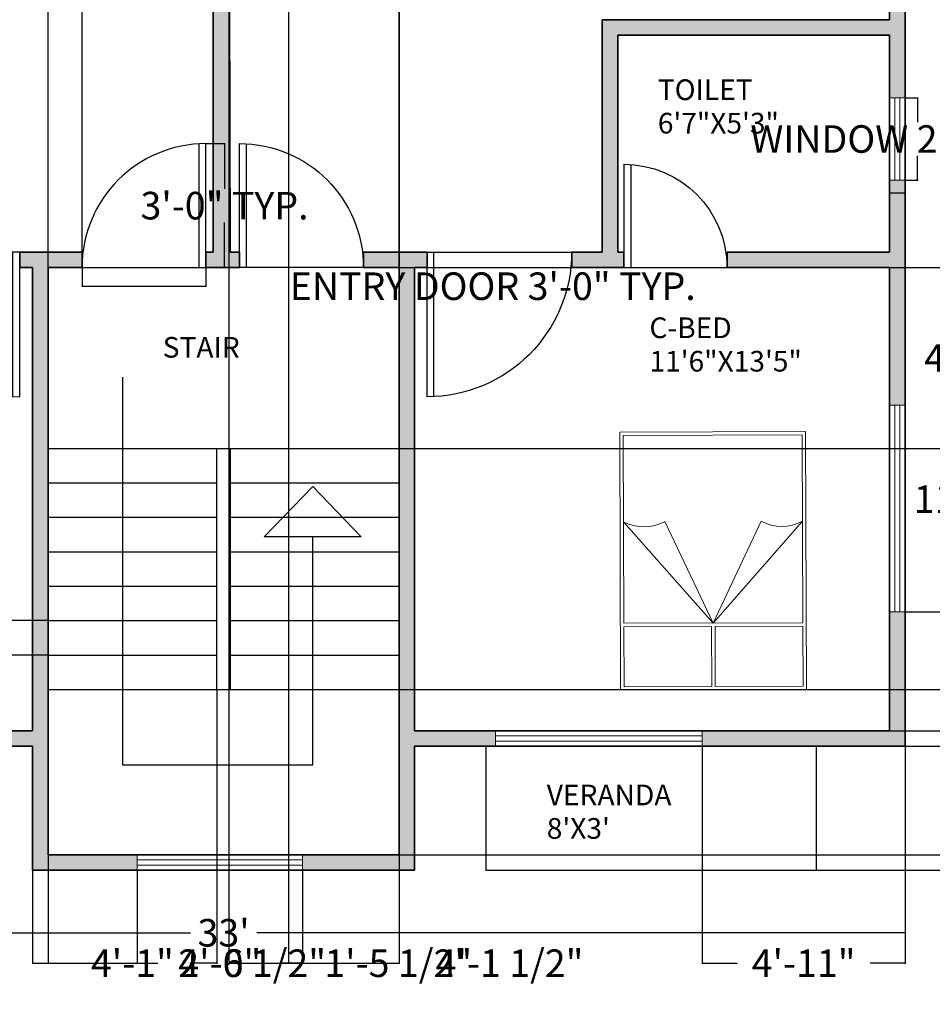
# Model space of a CAD drawing. Units: inches. Extents: x -27 to 662, y -19 to 539.
# Tile 2 of 4: x 160 to 425, y -19 to 267. Entities that reach past the tile are written whole.
import ezdxf

# ---------------------------------------------------------------- set-up
doc = ezdxf.new("R2010")
doc.units = ezdxf.units.IN
doc.header["$MEASUREMENT"] = 0
for name, color, linetype, lineweight in [('A-ANNO-DIMS', 2, 'Continuous', 18), ('A-AREA-IDEN', 230, 'Continuous', 18), ('A-DOOR', 6, 'Continuous', 25), ('A-FLOR', 4, 'Continuous', 25), ('A-FLOR-STRS', 5, 'Continuous', 25), ('A-FURN', 240, 'Continuous', 18), ('A-GLAZ', 240, 'Continuous', 18), ('A-WALL', 4, 'Continuous', 35)]:
    doc.layers.add(name, color=color, linetype=linetype, lineweight=lineweight)
doc.layers.add('A-WALL-PATT', color=2, linetype='Continuous', lineweight=13, true_color=0xf1eb1f)
doc.styles.get("Standard").update_dxf_attribs({"font": 'italic8.shx'})
doc.dimstyles.get("Standard").update_dxf_attribs({"dimtxt": 8, "dimasz": 0.18, "dimexe": 0.18, "dimexo": 0.0625, "dimgap": 0.09, "dimtad": 0, "dimtih": 1, "dimtoh": 1, "dimzin": 0, "dimdsep": 46, "dimlunit": 3, "dimtxsty": 'Standard', "dimcen": 0.09, "dimclrt": 4, "dimadec": 0, "dimazin": 0, "dimtfac": 1, "dimtofl": 0, "dimtmove": 0, "dimatfit": 3, "dimfxl": 1, "dimtolj": 1, "dimtzin": 0, "dimarcsym": 0})

# ---------------------------------------------------------------- blocks, each defined once
blk = doc.blocks.new('*D1')
at = {"layer": 'A-ANNO-DIMS', "color": 0, "lineweight": -2, "transparency": 16777216}
for p, q in [((21.29, 55.86), (21.29, 1.58)), ((417.29, 55.86), (417.29, 1.58)), ((21.47, 1.76), (209.67, 1.76)), ((417.11, 1.76), (228.9, 1.76))]:
    blk.add_line(p, q, dxfattribs=at)
at = {"layer": 'A-ANNO-DIMS', "color": 0, "transparency": 16777216}
for points in [[(21.47, 1.79), (21.47, 1.73), (21.29, 1.76)], [(417.11, 1.79), (417.11, 1.73), (417.29, 1.76)]]:
    blk.add_solid(points, dxfattribs=at)
at = {"layer": 'Defpoints', "color": 0, "transparency": 16777216}
for p in [(21.29, 55.92), (417.29, 55.92), (417.29, 1.76)]:
    blk.add_point(p, dxfattribs=at)
at = {"layer": 'A-ANNO-DIMS', "color": 0, "transparency": 16777216, "insert": (219.29, 1.76), "char_height": 8, "attachment_point": 5}
blk.add_mtext("\\A1;33'", dxfattribs=at)
blk = doc.blocks.new('*D2')
at = {"layer": 'A-ANNO-DIMS', "color": 0, "lineweight": -2, "transparency": 16777216}
for p, q in [((391.54, 495.42), (467.74, 495.42)), ((467.56, 495.24), (467.56, 262.52)), ((467.56, 20.1), (467.56, 252.82)), ((391.54, 19.92), (467.74, 19.92))]:
    blk.add_line(p, q, dxfattribs=at)
at = {"layer": 'A-ANNO-DIMS', "color": 0, "transparency": 16777216}
for points in [[(467.53, 495.24), (467.59, 495.24), (467.56, 495.42)], [(467.53, 20.1), (467.59, 20.1), (467.56, 19.92)]]:
    blk.add_solid(points, dxfattribs=at)
at = {"layer": 'Defpoints', "color": 0, "transparency": 16777216}
for p in [(391.48, 495.42), (467.56, 495.42), (391.48, 19.92)]:
    blk.add_point(p, dxfattribs=at)
at = {"layer": 'A-ANNO-DIMS', "color": 0, "transparency": 16777216, "insert": (467.56, 257.67), "char_height": 8, "attachment_point": 5}
blk.add_mtext('\\A1;39\'-7.50"', dxfattribs=at)
blk = doc.blocks.new('BED-DOUBLE-54x75')
for p, q in [((26.5, 56.54), (26.5, 74)), ((27.5, 56.54), (27.5, 74)), ((1, 56.54), (26.5, 56.54)), ((1, 55.54), (53, 55.54)), ((27, 55.54), (1, 26.04)), ((13, 26.04), (27, 55.54)), ((27, 55.54), (53, 26.04)), ((41, 26.04), (27, 55.54)), ((27.5, 56.54), (53, 56.54))]:
    blk.add_line(p, q)
blk.add_lwpolyline([(0, 75), (54, 75), (54, 0), (0, 0)], close=True)
for points in [[(1, 56.54), (1, 74), (26.5, 74)], [(27.5, 74), (53, 74), (53, 56.54)], [(53, 55.54), (53, 1), (1, 1), (1, 55.54)]]:
    blk.add_lwpolyline(points)
for centre in [(7, 14.92), (47, 14.92)]:
    blk.add_arc(centre, 12.64, 61.656, 118.344)
blk = doc.blocks.new('DOOR-SWING-30IN')
for p, q in [((28, 29.93), (28, 0)), ((30, 30), (30, 0)), ((30, 0), (0, 0))]:
    blk.add_line(p, q)
blk.add_arc((30, 0), 30, 90, 180)
blk = doc.blocks.new('DOOR-SWING-42IN')
for p, q in [((0, 42), (0, 0)), ((2, 41.95), (2, 0)), ((0, 0), (42, 0))]:
    blk.add_line(p, q)
blk.add_arc((0, 0), 42, 0, 90)
blk = doc.blocks.new('DOOR-SWING-36IN')
for p, q in [((34, 0), (34, 35.94)), ((36, 0), (36, 36)), ((0, 0), (36, 0))]:
    blk.add_line(p, q)
blk.add_arc((36, 0), 36, 90, 180)
blk = doc.blocks.new('WIN-60IN')
for p, q in [((0, 4.5), (0, 0)), ((60, 4.5), (0, 4.5)), ((0, 3), (60, 3)), ((60, 0), (60, 4.5)), ((0, 1.5), (60, 1.5)), ((0, 0), (60, 0))]:
    blk.add_line(p, q)
blk = doc.blocks.new('WIN-24IN-B')
for p, q in [((0, 24), (4.5, 24)), ((0, 0), (0, 24)), ((0, 24), (2.25, 24)), ((1.5, 24), (1.5, 0)), ((3, 24), (3, 0)), ((4.5, 24), (4.5, 0)), ((4.5, 0), (0, 0))]:
    blk.add_line(p, q)
blk = doc.blocks.new('*D18')
at = {"layer": 'A-ANNO-DIMS', "color": 0, "lineweight": -2, "transparency": 16777216}
for p, q in [((178.16, 194.86), (178.16, 189.34)), ((214.16, 194.86), (214.16, 189.34)), ((178.34, 189.52), (213.98, 189.52)), ((214.16, 189.52), (214.34, 189.52))]:
    blk.add_line(p, q, dxfattribs=at)
at = {"layer": 'A-ANNO-DIMS', "color": 0, "transparency": 16777216}
for points in [[(178.34, 189.55), (178.34, 189.49), (178.16, 189.52)], [(213.98, 189.55), (213.98, 189.49), (214.16, 189.52)]]:
    blk.add_solid(points, dxfattribs=at)
at = {"layer": 'Defpoints', "color": 0, "transparency": 16777216}
for p in [(178.16, 194.92), (214.16, 194.92), (214.16, 189.52)]:
    blk.add_point(p, dxfattribs=at)
at = {"layer": 'A-ANNO-DIMS', "color": 4, "transparency": 16777216, "insert": (297.48, 189.52), "char_height": 8, "attachment_point": 5}
blk.add_mtext('\\A1;ENTRY DOOR 3\'-0" TYP.', dxfattribs=at)
blk = doc.blocks.new('*D19')
at = {"layer": 'A-ANNO-DIMS', "color": 0, "lineweight": -2, "transparency": 16777216}
for p, q in [((214.23, 230.92), (219.74, 230.92)), ((219.56, 230.74), (219.56, 217.77)), ((219.56, 195.1), (219.56, 208.07)), ((214.23, 194.92), (219.74, 194.92))]:
    blk.add_line(p, q, dxfattribs=at)
at = {"layer": 'A-ANNO-DIMS', "color": 0, "transparency": 16777216}
for points in [[(219.53, 230.74), (219.59, 230.74), (219.56, 230.92)], [(219.53, 195.1), (219.59, 195.1), (219.56, 194.92)]]:
    blk.add_solid(points, dxfattribs=at)
at = {"layer": 'Defpoints', "color": 0, "transparency": 16777216}
for p in [(214.16, 230.92), (219.56, 230.92), (214.16, 194.92)]:
    blk.add_point(p, dxfattribs=at)
at = {"layer": 'A-ANNO-DIMS', "color": 4, "transparency": 16777216, "insert": (219.56, 212.92), "char_height": 8, "attachment_point": 5}
blk.add_mtext('\\A1;3\'-0" TYP.', dxfattribs=at)
blk = doc.blocks.new('*D26')
at = {"layer": 'A-ANNO-DIMS', "color": 0, "lineweight": -2, "transparency": 16777216}
for p, q in [((417.35, 244.27), (421.07, 244.27)), ((420.89, 244.09), (420.89, 237.12)), ((420.89, 220.45), (420.89, 227.42)), ((417.35, 220.27), (421.07, 220.27))]:
    blk.add_line(p, q, dxfattribs=at)
at = {"layer": 'A-ANNO-DIMS', "color": 0, "transparency": 16777216}
for points in [[(420.86, 244.09), (420.92, 244.09), (420.89, 244.27)], [(420.86, 220.45), (420.92, 220.45), (420.89, 220.27)]]:
    blk.add_solid(points, dxfattribs=at)
at = {"layer": 'Defpoints', "color": 0, "transparency": 16777216}
for p in [(417.29, 244.27), (420.89, 244.27), (417.29, 220.27)]:
    blk.add_point(p, dxfattribs=at)
at = {"layer": 'A-ANNO-DIMS', "color": 4, "transparency": 16777216, "insert": (420.89, 232.27), "char_height": 8, "attachment_point": 5}
blk.add_mtext('\\A1;WINDOW 2\'-0" TYP.', dxfattribs=at)
blk = doc.blocks.new('*D27')
at = {"layer": 'A-ANNO-DIMS', "color": 0, "lineweight": -2, "transparency": 16777216}
for p, q in [((412.79, 220.21), (412.79, 216.49)), ((417.29, 220.21), (417.29, 216.49)), ((412.97, 216.67), (417.11, 216.67)), ((417.29, 216.67), (417.47, 216.67))]:
    blk.add_line(p, q, dxfattribs=at)
at = {"layer": 'A-ANNO-DIMS', "color": 0, "transparency": 16777216}
for points in [[(412.97, 216.7), (412.97, 216.64), (412.79, 216.67)], [(417.11, 216.7), (417.11, 216.64), (417.29, 216.67)]]:
    blk.add_solid(points, dxfattribs=at)
at = {"layer": 'Defpoints', "color": 0, "transparency": 16777216}
for p in [(412.79, 220.27), (417.29, 220.27), (417.29, 216.67)]:
    blk.add_point(p, dxfattribs=at)
at = {"layer": 'A-ANNO-DIMS', "color": 4, "transparency": 16777216, "insert": (468.99, 216.67), "char_height": 8, "attachment_point": 5}
blk.add_mtext('\\A1;0\'-4 1/2" TYP.', dxfattribs=at)
blk = doc.blocks.new('*D30')
at = {"layer": 'A-ANNO-DIMS', "color": 0, "lineweight": -2, "transparency": 16777216}
for p, q in [((417.35, 499.92), (444.47, 499.92)), ((444.29, 499.74), (444.29, 264.77)), ((444.29, 20.1), (444.29, 255.07)), ((391.54, 19.92), (444.47, 19.92))]:
    blk.add_line(p, q, dxfattribs=at)
at = {"layer": 'A-ANNO-DIMS', "color": 0, "transparency": 16777216}
for points in [[(444.26, 499.74), (444.32, 499.74), (444.29, 499.92)], [(444.26, 20.1), (444.32, 20.1), (444.29, 19.92)]]:
    blk.add_solid(points, dxfattribs=at)
at = {"layer": 'Defpoints', "color": 0, "transparency": 16777216}
for p in [(417.29, 499.92), (444.29, 499.92), (391.48, 19.92)]:
    blk.add_point(p, dxfattribs=at)
at = {"layer": 'A-ANNO-DIMS', "color": 4, "transparency": 16777216, "insert": (444.29, 259.92), "char_height": 8, "attachment_point": 5}
blk.add_mtext('\\A1;40\'-0"', dxfattribs=at)
blk = doc.blocks.new('*D31')
at = {"layer": 'A-ANNO-DIMS', "color": 0, "lineweight": -2, "transparency": 16777216}
for p, q in [((168.29, 142.48), (168.29, 527.1)), ((168.47, 526.92), (201.29, 526.92)), ((270.11, 526.92), (237.28, 526.92)), ((270.29, 142.48), (270.29, 527.1))]:
    blk.add_line(p, q, dxfattribs=at)
at = {"layer": 'A-ANNO-DIMS', "color": 0, "transparency": 16777216}
for points in [[(168.47, 526.95), (168.47, 526.89), (168.29, 526.92)], [(270.11, 526.95), (270.11, 526.89), (270.29, 526.92)]]:
    blk.add_solid(points, dxfattribs=at)
at = {"layer": 'Defpoints', "color": 0, "transparency": 16777216}
for p in [(270.29, 526.92), (168.29, 142.42), (270.29, 142.42)]:
    blk.add_point(p, dxfattribs=at)
at = {"layer": 'A-ANNO-DIMS', "color": 4, "transparency": 16777216, "insert": (219.29, 526.92), "char_height": 8, "attachment_point": 5}
blk.add_mtext('\\A1;8\'-6"', dxfattribs=at)
blk = doc.blocks.new('*D32')
at = {"layer": 'A-ANNO-DIMS', "color": 0, "lineweight": -2, "transparency": 16777216}
for p, q in [((270.35, 142.42), (444.47, 142.42)), ((444.29, 142.24), (444.29, 112.27)), ((444.29, 72.6), (444.29, 102.57)), ((270.35, 72.42), (444.47, 72.42))]:
    blk.add_line(p, q, dxfattribs=at)
at = {"layer": 'A-ANNO-DIMS', "color": 0, "transparency": 16777216}
for points in [[(444.26, 142.24), (444.32, 142.24), (444.29, 142.42)], [(444.26, 72.6), (444.32, 72.6), (444.29, 72.42)]]:
    blk.add_solid(points, dxfattribs=at)
at = {"layer": 'Defpoints', "color": 0, "transparency": 16777216}
for p in [(270.29, 142.42), (444.29, 142.42), (270.29, 72.42)]:
    blk.add_point(p, dxfattribs=at)
at = {"layer": 'A-ANNO-DIMS', "color": 4, "transparency": 16777216, "insert": (444.29, 107.42), "char_height": 8, "attachment_point": 5}
blk.add_mtext('\\A1;5\'-10"', dxfattribs=at)
blk = doc.blocks.new('*D33')
at = {"layer": 'A-ANNO-DIMS', "color": 0, "lineweight": -2, "transparency": 16777216}
for p, q in [((270.35, 194.92), (444.47, 194.92)), ((444.29, 194.74), (444.29, 174.85)), ((444.29, 142.6), (444.29, 162.48)), ((270.35, 142.42), (444.47, 142.42))]:
    blk.add_line(p, q, dxfattribs=at)
at = {"layer": 'A-ANNO-DIMS', "color": 0, "transparency": 16777216}
for points in [[(444.26, 194.74), (444.32, 194.74), (444.29, 194.92)], [(444.26, 142.6), (444.32, 142.6), (444.29, 142.42)]]:
    blk.add_solid(points, dxfattribs=at)
at = {"layer": 'Defpoints', "color": 0, "transparency": 16777216}
for p in [(270.29, 194.92), (444.29, 194.92), (270.29, 142.42)]:
    blk.add_point(p, dxfattribs=at)
at = {"layer": 'A-ANNO-DIMS', "color": 4, "transparency": 16777216, "insert": (444.29, 168.67), "char_height": 8, "attachment_point": 5}
blk.add_mtext('\\A1;4\'-4 1/2"', dxfattribs=at)
blk = doc.blocks.new('*D34')
at = {"layer": 'A-ANNO-DIMS', "color": 0, "lineweight": -2, "transparency": 16777216}
for p, q in [((270.35, 72.42), (444.47, 72.42)), ((444.29, 72.24), (444.29, 53.27)), ((444.29, 24.6), (444.29, 43.57)), ((270.35, 24.42), (444.47, 24.42))]:
    blk.add_line(p, q, dxfattribs=at)
at = {"layer": 'A-ANNO-DIMS', "color": 0, "transparency": 16777216}
for points in [[(444.26, 72.24), (444.32, 72.24), (444.29, 72.42)], [(444.26, 24.6), (444.32, 24.6), (444.29, 24.42)]]:
    blk.add_solid(points, dxfattribs=at)
at = {"layer": 'Defpoints', "color": 0, "transparency": 16777216}
for p in [(270.29, 72.42), (444.29, 72.42), (270.29, 24.42)]:
    blk.add_point(p, dxfattribs=at)
at = {"layer": 'A-ANNO-DIMS', "color": 4, "transparency": 16777216, "insert": (444.29, 48.42), "char_height": 8, "attachment_point": 5}
blk.add_mtext('\\A1;4\'-0"', dxfattribs=at)
blk = doc.blocks.new('*D35')
at = {"layer": 'A-ANNO-DIMS', "color": 0, "lineweight": -2, "transparency": 16777216}
for p, q in [((168.29, 72.36), (168.29, -7.26)), ((217.29, 72.36), (217.29, -7.26)), ((168.47, -7.08), (176.13, -7.08)), ((217.11, -7.08), (209.45, -7.08))]:
    blk.add_line(p, q, dxfattribs=at)
at = {"layer": 'A-ANNO-DIMS', "color": 0, "transparency": 16777216}
for points in [[(168.47, -7.05), (168.47, -7.11), (168.29, -7.08)], [(217.11, -7.05), (217.11, -7.11), (217.29, -7.08)]]:
    blk.add_solid(points, dxfattribs=at)
at = {"layer": 'Defpoints', "color": 0, "transparency": 16777216}
for p in [(168.29, 72.42), (217.29, 72.42), (217.29, -7.08)]:
    blk.add_point(p, dxfattribs=at)
at = {"layer": 'A-ANNO-DIMS', "color": 4, "transparency": 16777216, "insert": (192.79, -7.08), "char_height": 8, "attachment_point": 5}
blk.add_mtext('\\A1;4\'-1"', dxfattribs=at)
blk = doc.blocks.new('*D36')
at = {"layer": 'A-ANNO-DIMS', "color": 0, "lineweight": -2, "transparency": 16777216}
for p, q in [((168.225254, 92.419463), (-5.892246, 92.419463)), ((-5.712246, 92.599463), (-5.712246, 92.779463)), ((168.225254, 82.419463), (-5.892246, 82.419463)), ((-5.712246, 82.239463), (-5.712246, 82.059463))]:
    blk.add_line(p, q, dxfattribs=at)
at = {"layer": 'A-ANNO-DIMS', "color": 0, "transparency": 16777216}
for points in [[(-5.742246, 92.599463), (-5.682246, 92.599463), (-5.712246, 92.419463)], [(-5.742246, 82.239463), (-5.682246, 82.239463), (-5.712246, 82.419463)]]:
    blk.add_solid(points, dxfattribs=at)
at = {"layer": 'Defpoints', "color": 0, "transparency": 16777216}
for p in [(-5.712246, 92.419463), (168.287754, 92.419463), (168.287754, 82.419463)]:
    blk.add_point(p, dxfattribs=at)
at = {"layer": 'A-ANNO-DIMS', "color": 4, "transparency": 16777216, "insert": (-5.712246, 87.419463), "char_height": 8, "attachment_point": 5}
blk.add_mtext('\\A1;0\'-10"', dxfattribs=at)
blk = doc.blocks.new('*D37')
at = {"layer": 'A-ANNO-DIMS', "color": 0, "lineweight": -2, "transparency": 16777216}
for p, q in [((194.19, 19.86), (194.19, -7.26)), ((242.19, 19.86), (242.19, -7.26)), ((194.37, -7.08), (200.19, -7.08)), ((242.01, -7.08), (236.18, -7.08))]:
    blk.add_line(p, q, dxfattribs=at)
at = {"layer": 'A-ANNO-DIMS', "color": 0, "transparency": 16777216}
for points in [[(194.37, -7.05), (194.37, -7.11), (194.19, -7.08)], [(242.01, -7.05), (242.01, -7.11), (242.19, -7.08)]]:
    blk.add_solid(points, dxfattribs=at)
at = {"layer": 'Defpoints', "color": 0, "transparency": 16777216}
for p in [(194.19, 19.92), (242.19, 19.92), (242.19, -7.08)]:
    blk.add_point(p, dxfattribs=at)
at = {"layer": 'A-ANNO-DIMS', "color": 4, "transparency": 16777216, "insert": (218.19, -7.08), "char_height": 8, "attachment_point": 5}
blk.add_mtext('\\A1;4\'-0"', dxfattribs=at)
blk = doc.blocks.new('*D38')
at = {"layer": 'A-ANNO-DIMS', "color": 0, "lineweight": -2, "transparency": 16777216}
for p, q in [((163.79, 19.86), (163.79, -7.26)), ((194.19, 19.86), (194.19, -7.26)), ((163.97, -7.08), (194.01, -7.08)), ((194.19, -7.08), (194.37, -7.08))]:
    blk.add_line(p, q, dxfattribs=at)
at = {"layer": 'A-ANNO-DIMS', "color": 0, "transparency": 16777216}
for points in [[(163.97, -7.05), (163.97, -7.11), (163.79, -7.08)], [(194.01, -7.05), (194.01, -7.11), (194.19, -7.08)]]:
    blk.add_solid(points, dxfattribs=at)
at = {"layer": 'Defpoints', "color": 0, "transparency": 16777216}
for p in [(163.79, 19.92), (194.19, 19.92), (194.19, -7.08)]:
    blk.add_point(p, dxfattribs=at)
at = {"layer": 'A-ANNO-DIMS', "color": 4, "transparency": 16777216, "insert": (227.6, -7.08), "char_height": 8, "attachment_point": 5}
blk.add_mtext('\\A1;2\'-6 1/2"', dxfattribs=at)
blk = doc.blocks.new('*D39')
at = {"layer": 'A-ANNO-DIMS', "color": 0, "lineweight": -2, "transparency": 16777216}
for p, q in [((168.29, 194.98), (168.29, 527.1)), ((168.47, 526.92), (177.98, 526.92)), ((178.16, 194.98), (178.16, 527.1)), ((178.16, 526.92), (178.34, 526.92))]:
    blk.add_line(p, q, dxfattribs=at)
at = {"layer": 'A-ANNO-DIMS', "color": 0, "transparency": 16777216}
for points in [[(168.47, 526.95), (168.47, 526.89), (168.29, 526.92)], [(177.98, 526.95), (177.98, 526.89), (178.16, 526.92)]]:
    blk.add_solid(points, dxfattribs=at)
at = {"layer": 'Defpoints', "color": 0, "transparency": 16777216}
for p in [(178.16, 526.92), (168.29, 194.92), (178.16, 194.92)]:
    blk.add_point(p, dxfattribs=at)
at = {"layer": 'A-ANNO-DIMS', "color": 4, "transparency": 16777216, "insert": (199, 526.92), "char_height": 8, "attachment_point": 5}
blk.add_mtext('\\A1;0\'-10"', dxfattribs=at)
blk = doc.blocks.new('*D40')
at = {"layer": 'A-ANNO-DIMS', "color": 0, "lineweight": -2, "transparency": 16777216}
for p, q in [((412.85, 194.92), (444.47, 194.92)), ((444.29, 194.74), (444.29, 133.85)), ((444.29, 60.6), (444.29, 121.48)), ((412.85, 60.42), (444.47, 60.42))]:
    blk.add_line(p, q, dxfattribs=at)
at = {"layer": 'A-ANNO-DIMS', "color": 0, "transparency": 16777216}
for points in [[(444.26, 194.74), (444.32, 194.74), (444.29, 194.92)], [(444.26, 60.6), (444.32, 60.6), (444.29, 60.42)]]:
    blk.add_solid(points, dxfattribs=at)
at = {"layer": 'Defpoints', "color": 0, "transparency": 16777216}
for p in [(412.79, 194.92), (444.29, 194.92), (412.79, 60.42)]:
    blk.add_point(p, dxfattribs=at)
at = {"layer": 'A-ANNO-DIMS', "color": 4, "transparency": 16777216, "insert": (444.29, 127.67), "char_height": 8, "attachment_point": 5}
blk.add_mtext('\\A1;11\'-2 1/2"', dxfattribs=at)
blk = doc.blocks.new('*D51')
at = {"layer": 'A-ANNO-DIMS', "color": 0, "lineweight": -2, "transparency": 16777216}
for p, q in [((417.35, 94.96), (444.47, 94.96)), ((444.29, 94.78), (444.29, 80.29)), ((444.29, 56.1), (444.29, 70.59)), ((417.35, 55.92), (444.47, 55.92))]:
    blk.add_line(p, q, dxfattribs=at)
at = {"layer": 'A-ANNO-DIMS', "color": 0, "transparency": 16777216}
for points in [[(444.26, 94.78), (444.32, 94.78), (444.29, 94.96)], [(444.26, 56.1), (444.32, 56.1), (444.29, 55.92)]]:
    blk.add_solid(points, dxfattribs=at)
at = {"layer": 'Defpoints', "color": 0, "transparency": 16777216}
for p in [(417.29, 94.96), (444.29, 94.96), (417.29, 55.92)]:
    blk.add_point(p, dxfattribs=at)
at = {"layer": 'A-ANNO-DIMS', "color": 4, "transparency": 16777216, "insert": (444.29, 75.44), "char_height": 8, "attachment_point": 5}
blk.add_mtext('\\A1;3\'-3"', dxfattribs=at)
blk = doc.blocks.new('*D52')
at = {"layer": 'A-ANNO-DIMS', "color": 0, "lineweight": -2, "transparency": 16777216}
for p, q in [((358.32, 55.86), (358.32, -7.26)), ((417.29, 55.86), (417.29, -7.26)), ((358.5, -7.08), (368.48, -7.08)), ((417.11, -7.08), (407.13, -7.08))]:
    blk.add_line(p, q, dxfattribs=at)
at = {"layer": 'A-ANNO-DIMS', "color": 0, "transparency": 16777216}
for points in [[(358.5, -7.05), (358.5, -7.11), (358.32, -7.08)], [(417.11, -7.05), (417.11, -7.11), (417.29, -7.08)]]:
    blk.add_solid(points, dxfattribs=at)
at = {"layer": 'Defpoints', "color": 0, "transparency": 16777216}
for p in [(358.32, 55.92), (417.29, 55.92), (417.29, -7.08)]:
    blk.add_point(p, dxfattribs=at)
at = {"layer": 'A-ANNO-DIMS', "color": 4, "transparency": 16777216, "insert": (387.8, -7.08), "char_height": 8, "attachment_point": 5}
blk.add_mtext('\\A1;4\'-11"', dxfattribs=at)
blk = doc.blocks.new('*D54')
at = {"layer": 'A-ANNO-DIMS', "color": 0, "lineweight": -2, "transparency": 16777216}
for p, q in [((220.8, 406.86), (220.8, -7.26)), ((238.14, 406.86), (238.14, -7.26)), ((220.98, -7.08), (237.96, -7.08)), ((238.14, -7.08), (238.32, -7.08))]:
    blk.add_line(p, q, dxfattribs=at)
at = {"layer": 'A-ANNO-DIMS', "color": 0, "transparency": 16777216}
for points in [[(220.98, -7.05), (220.98, -7.11), (220.8, -7.08)], [(237.96, -7.05), (237.96, -7.11), (238.14, -7.08)]]:
    blk.add_solid(points, dxfattribs=at)
at = {"layer": 'Defpoints', "color": 0, "transparency": 16777216}
for p in [(220.8, 406.92), (238.14, 406.92), (238.14, -7.08)]:
    blk.add_point(p, dxfattribs=at)
at = {"layer": 'A-ANNO-DIMS', "color": 4, "transparency": 16777216, "insert": (270.03, -7.08), "char_height": 8, "attachment_point": 5}
blk.add_mtext('\\A1;1\'-5 1/2"', dxfattribs=at)
blk = doc.blocks.new('*D58')
at = {"layer": 'A-ANNO-DIMS', "color": 0, "lineweight": -2, "transparency": 16777216}
for p, q in [((220.79, 495.36), (220.79, -7.26)), ((270.29, 495.36), (270.29, -7.26)), ((220.97, -7.08), (270.11, -7.08)), ((270.29, -7.08), (270.47, -7.08))]:
    blk.add_line(p, q, dxfattribs=at)
at = {"layer": 'A-ANNO-DIMS', "color": 0, "transparency": 16777216}
for points in [[(220.97, -7.05), (220.97, -7.11), (220.79, -7.08)], [(270.11, -7.05), (270.11, -7.11), (270.29, -7.08)]]:
    blk.add_solid(points, dxfattribs=at)
at = {"layer": 'Defpoints', "color": 0, "transparency": 16777216}
for p in [(220.79, 495.42), (270.29, 495.42), (270.29, -7.08)]:
    blk.add_point(p, dxfattribs=at)
at = {"layer": 'A-ANNO-DIMS', "color": 4, "transparency": 16777216, "insert": (302.37, -7.08), "char_height": 8, "attachment_point": 5}
blk.add_mtext('\\A1;4\'-1 1/2"', dxfattribs=at)

msp = doc.modelspace()

# ---------------------------------------------------------------- hatches: boundary and pattern name
at = {"layer": 'A-WALL-PATT'}
h = msp.add_hatch(color=256, dxfattribs=at)
h.dxf.hatch_style = 1
h.paths.add_polyline_path([(79.868, 60.419), (25.788, 60.419), (25.788, 105.383), (21.288, 105.383), (21.288, 55.919), (79.868, 55.919)])
h.paths.add_polyline_path([(168.288, 194.919), (178.163, 194.919), (178.163, 199.419), (160.053, 199.419), (160.053, 194.919), (163.788, 194.919), (163.788, 60.419), (139.868, 60.419), (139.868, 58.169), (139.868, 55.919), (163.788, 55.919), (163.788, 19.919), (194.188, 19.919), (194.188, 24.419), (168.288, 24.419)])
h.paths.add_polyline_path([(298.321, 60.419), (274.788, 60.419), (274.788, 194.919), (278.414, 194.919), (278.414, 199.419), (270.288, 199.419), (259.929, 199.419), (259.929, 194.919), (270.288, 194.919), (270.288, 24.419), (242.188, 24.419), (242.188, 19.919), (274.788, 19.919), (274.788, 55.919), (298.321, 55.919)])
h.paths.add_polyline_path([(417.288, 94.965), (412.788, 94.965), (412.788, 60.419), (358.321, 60.419), (358.321, 55.919), (417.288, 55.919)])
h.paths.add_polyline_path([(417.288, 220.271), (412.788, 220.271), (412.788, 199.419), (365.562, 199.419), (365.562, 194.919), (412.788, 194.919), (412.788, 154.965), (417.288, 154.965)])
h.paths.add_polyline_path([(333.788, 262.419), (412.788, 262.419), (412.788, 244.271), (415.038, 244.271), (417.288, 244.271), (417.288, 283.252), (412.788, 283.252), (412.788, 266.919), (329.288, 266.919), (329.288, 262.419), (329.288, 199.419), (320.414, 199.419), (320.414, 194.919), (335.562, 194.919), (335.562, 199.419), (333.788, 199.419)])
h.paths.add_polyline_path([(333.788, 329.919), (412.788, 329.919), (412.788, 319.252), (415.038, 319.252), (417.288, 319.252), (417.288, 356.883), (415.038, 356.883), (412.788, 356.883), (412.788, 334.419), (320.72, 334.419), (320.72, 329.919), (329.288, 329.919), (329.288, 297.07), (333.788, 297.07)])
h.paths.add_polyline_path([(220.796, 406.919), (238.139, 406.919), (238.139, 411.419), (220.788, 411.419), (220.788, 495.419), (229.602, 495.419), (229.602, 499.919), (203.089, 499.919), (203.089, 495.419), (216.288, 495.419), (216.288, 411.419), (200.507, 411.419), (200.507, 406.919), (216.288, 406.919), (216.288, 199.419), (214.163, 199.419), (214.163, 194.919), (223.929, 194.919), (223.929, 199.419), (221.182, 199.419)])
h.paths.add_polyline_path([(109.288, 266.919), (104.788, 266.919), (25.788, 266.919), (25.788, 262.419), (104.788, 262.419), (104.788, 199.419), (101.522, 199.419), (101.522, 194.919), (118.053, 194.919), (118.053, 199.419), (109.288, 199.419)])
h.paths.add_polyline_path([(71.522, 199.419), (25.788, 199.419), (25.788, 220.271), (21.288, 220.271), (21.288, 165.383), (25.788, 165.383), (25.788, 194.919), (71.522, 194.919)])
h.paths.add_polyline_path([(25.788, 283.252), (21.288, 283.252), (21.288, 244.271), (23.538, 244.271), (25.788, 244.271)])
h.paths.add_polyline_path([(118.822, 334.419), (25.788, 334.419), (25.788, 495.419), (61.341, 495.419), (61.341, 499.919), (21.288, 499.919), (21.288, 319.252), (23.538, 319.252), (25.788, 319.252), (25.788, 329.919), (104.788, 329.919), (104.788, 296.919), (109.288, 296.919), (109.288, 329.919), (118.822, 329.919)])
h.paths.add_polyline_path([(168.288, 406.919), (170.507, 406.919), (170.507, 411.419), (168.288, 411.419), (168.288, 495.419), (179.089, 495.419), (179.089, 499.919), (121.341, 499.919), (121.341, 495.419), (163.788, 495.419), (163.788, 334.419), (160.822, 334.419), (160.822, 329.919), (168.288, 329.919)])
h.paths.add_polyline_path([(312.716, 499.919), (253.602, 499.919), (253.602, 495.419), (270.288, 495.419), (270.288, 411.419), (268.139, 411.419), (268.139, 406.919), (270.288, 406.919), (270.288, 329.919), (278.72, 329.919), (278.72, 334.419), (274.788, 334.419), (274.788, 495.419), (312.716, 495.419)])
h.paths.add_polyline_path([(417.288, 499.919), (372.716, 499.919), (372.716, 495.419), (412.788, 495.419), (412.788, 416.883), (417.288, 416.883)])

# ---------------------------------------------------------------- linework, layer by layer
at = {"layer": 'A-FLOR'}
for p, q in [((295.48, 55.919), (295.48, 19.919)), ((391.48, 55.919), (391.48, 19.919)), ((295.48, 19.919), (391.48, 19.919))]:
    msp.add_line(p, q, dxfattribs=at)
at = {"layer": 'A-FLOR-STRS'}
for p, q in [((189.912, 163.15), (189.912, 50.507)), ((168.288, 142.419), (270.288, 142.419)), ((217.288, 72.419), (217.288, 142.419)), ((221.288, 72.419), (221.288, 142.419)), ((168.288, 132.419), (217.288, 132.419)), ((221.288, 132.419), (270.288, 132.419)), ((231.088, 116.78), (245.175, 131.377)), ((259.263, 116.78), (245.175, 131.377)), ((168.288, 122.419), (217.288, 122.419)), ((221.288, 122.419), (270.288, 122.419)), ((259.263, 116.78), (231.088, 116.78)), ((245.175, 50.507), (245.175, 116.78)), ((168.288, 112.419), (217.288, 112.419)), ((221.288, 112.419), (270.288, 112.419)), ((168.288, 102.419), (217.288, 102.419)), ((221.288, 102.419), (270.288, 102.419)), ((168.288, 92.419), (217.288, 92.419)), ((221.288, 92.419), (270.288, 92.419)), ((168.288, 82.419), (217.288, 82.419)), ((221.288, 82.419), (270.288, 82.419)), ((168.288, 72.419), (270.288, 72.419)), ((189.912, 50.507), (245.175, 50.507))]:
    msp.add_line(p, q, dxfattribs=at)
at = {"layer": 'A-GLAZ'}
for p, q in [((194.188, 24.419), (194.188, 19.919)), ((242.188, 24.419), (194.188, 24.419)), ((194.188, 22.919), (242.188, 22.919)), ((242.188, 19.919), (242.188, 24.419)), ((194.188, 21.419), (242.188, 21.419)), ((194.188, 19.919), (242.188, 19.919))]:
    msp.add_line(p, q, dxfattribs=at)
at = {"layer": 'A-WALL'}
for p, q in [((417.288, 55.919), (417.288, 499.919)), ((216.288, 406.919), (216.288, 199.419)), ((220.796, 406.919), (221.182, 199.419)), ((412.788, 266.919), (412.788, 329.919)), ((412.788, 266.919), (329.288, 266.919)), ((329.288, 262.419), (329.288, 266.919)), ((329.288, 199.419), (329.288, 262.419)), ((412.788, 262.419), (333.788, 262.419)), ((333.788, 199.419), (333.788, 262.419)), ((412.788, 199.419), (412.788, 262.419)), ((178.163, 199.419), (160.053, 199.419)), ((160.053, 199.419), (160.053, 194.919)), ((178.163, 199.419), (178.163, 194.919)), ((216.288, 199.419), (214.163, 199.419)), ((214.163, 199.419), (214.163, 194.919)), ((223.929, 199.419), (221.182, 199.419)), ((223.929, 199.419), (223.929, 194.919)), ((270.288, 199.419), (259.929, 199.419)), ((259.929, 199.419), (259.929, 194.919)), ((278.414, 199.419), (270.288, 199.419)), ((278.414, 199.419), (278.414, 194.919)), ((329.288, 199.419), (320.414, 199.419)), ((320.414, 199.419), (320.414, 194.919)), ((335.562, 199.419), (333.788, 199.419)), ((335.562, 199.419), (335.562, 194.919)), ((412.788, 199.419), (365.562, 199.419)), ((365.562, 199.419), (365.562, 194.919)), ((163.788, 194.919), (160.053, 194.919)), ((163.788, 194.919), (163.788, 60.419)), ((168.288, 194.919), (168.288, 24.419)), ((178.163, 194.919), (168.288, 194.919)), ((223.929, 194.919), (214.163, 194.919)), ((270.288, 194.919), (259.929, 194.919)), ((270.288, 24.419), (270.288, 194.919)), ((274.788, 60.419), (274.788, 194.919)), ((278.414, 194.919), (274.788, 194.919)), ((335.562, 194.919), (320.414, 194.919)), ((412.788, 194.919), (365.562, 194.919)), ((412.788, 60.419), (412.788, 194.919)), ((25.788, 60.419), (163.788, 60.419)), ((274.788, 60.419), (412.788, 60.419)), ((21.288, 55.919), (163.788, 55.919)), ((163.788, 55.919), (163.788, 19.919)), ((274.788, 19.919), (274.788, 55.919)), ((274.788, 55.919), (417.288, 55.919)), ((168.288, 24.419), (270.288, 24.419)), ((163.788, 19.919), (274.788, 19.919))]:
    msp.add_line(p, q, dxfattribs=at)

# ---------------------------------------------------------------- block references
at = {"layer": 'A-DOOR'}
msp.add_blockref('DOOR-SWING-36IN', (178.163, 194.919), dxfattribs=at)
at = {"layer": 'A-DOOR', "extrusion": (0, 0, -1), "zscale": -1}
for name, p in [('DOOR-SWING-36IN', (-259.929, 194.919)), ('DOOR-SWING-30IN', (-365.563, 194.919))]:
    msp.add_blockref(name, p, dxfattribs=at)
at = {"layer": 'A-DOOR', "rotation": 180}
msp.add_blockref('DOOR-SWING-42IN', (160.053, 199.42), dxfattribs=at)
at = {"layer": 'A-DOOR', "extrusion": (0, 0, -1), "zscale": -1, "rotation": 180}
msp.add_blockref('DOOR-SWING-42IN', (-278.415, 199.42), dxfattribs=at)
at = {"layer": 'A-FURN', "rotation": 180.1904805262934}
msp.add_blockref('BED-DOUBLE-54x75', (388.37, 147.347), dxfattribs=at)
at = {"layer": 'A-GLAZ'}
msp.add_blockref('WIN-24IN-B', (412.788, 220.271), dxfattribs=at)
for p, rotation in [((412.787, 154.965), 269.9999999999998), ((358.321, 60.42), 180)]:
    msp.add_blockref('WIN-60IN', p, dxfattribs=dict(at, rotation=rotation))

# ---------------------------------------------------------------- texts
at = {"layer": 'A-AREA-IDEN'}
for s, p in [('TOILET', (345.435, 243.581)), ('6\'7"X5\'3"', (345.435, 233.867)), ('C-BED', (343.006, 174.451)), ('STAIR', (201.608, 168.779)), ('11\'6"X13\'5"', (343.006, 164.737)), ('VERANDA', (313.176, 38.78)), ("8'X3'", (313.176, 29.066))]:
    msp.add_text(s, height=6, dxfattribs=at).set_placement(p)

# ---------------------------------------------------------------- dimensions: what is measured, and where the dimension line sits
at = {"layer": 'A-ANNO-DIMS'}
for base, p1, p2, override, picture, middle in [((270.288, 526.919), (168.288, 142.419), (270.288, 142.419), {"dimdec": 1, "dimlfac": 1, "dimrnd": 0, "dimzin": 1, "dimdsep": 46, "dimlunit": 4, "dimfrac": 2}, '*D31', (219.288, 526.919)), ((178.163, 526.919), (168.288, 194.919), (178.163, 194.919), {"dimdec": 1, "dimlfac": 1, "dimrnd": 0, "dimzin": 1, "dimdsep": 46, "dimlunit": 4, "dimfrac": 2}, '*D39', (199.004, 526.919)), ((270.288, -7.081), (220.788, 495.419), (270.288, 495.419), {"dimdec": 1, "dimlfac": 1, "dimrnd": 0, "dimzin": 1, "dimdsep": 46, "dimlunit": 4, "dimfrac": 2}, '*D58', (302.367, -7.081)), ((238.139, -7.081), (220.796, 406.919), (238.139, 406.919), {"dimdec": 1, "dimlfac": 1, "dimrnd": 0, "dimzin": 1, "dimdsep": 46, "dimlunit": 4, "dimfrac": 2}, '*D54', (270.028, -7.081)), ((217.288, -7.081), (168.288, 72.419), (217.288, 72.419), {"dimdec": 1, "dimlfac": 1, "dimrnd": 0, "dimzin": 1, "dimdsep": 46, "dimlunit": 4, "dimfrac": 2}, '*D35', (192.788, -7.081)), ((417.288, 1.759), (21.288, 55.919), (417.288, 55.919), {"dimclrd": 0, "dimclre": 0, "dimclrt": 0}, '*D1', (219.288, 1.759)), ((417.288, -7.081), (358.321, 55.919), (417.288, 55.919), {"dimdec": 1, "dimlfac": 1, "dimrnd": 0, "dimzin": 1, "dimdsep": 46, "dimlunit": 4, "dimfrac": 2}, '*D52', (387.804, -7.081)), ((194.188, -7.081), (163.788, 19.919), (194.188, 19.919), {"dimdec": 1, "dimlfac": 1, "dimrnd": 0, "dimzin": 1, "dimdsep": 46, "dimlunit": 4, "dimfrac": 2}, '*D38', (227.601, -7.081)), ((242.188, -7.081), (194.188, 19.919), (242.188, 19.919), {"dimdec": 1, "dimlfac": 1, "dimrnd": 0, "dimzin": 1, "dimdsep": 46, "dimlunit": 4, "dimfrac": 2}, '*D37', (218.188, -7.081))]:
    dim = msp.add_linear_dim(base=base, p1=p1, p2=p2, dimstyle='Standard', override=override, dxfattribs=at)
    dim.commit()
    dim.dimension.update_dxf_attribs({"geometry": picture, "text_midpoint": middle})
for base, p1, p2, override, picture, middle in [((444.288, 499.919), (391.48, 19.919), (417.288, 499.919), {"dimdec": 1, "dimlfac": 1, "dimrnd": 0, "dimzin": 1, "dimdsep": 46, "dimlunit": 4, "dimfrac": 2}, '*D30', (444.288, 259.919)), ((467.557, 495.419), (391.48, 19.919), (391.48, 495.419), {"dimclrd": 0, "dimclre": 0, "dimclrt": 0}, '*D2', (467.557, 257.669)), ((444.288, 194.919), (270.288, 142.419), (270.288, 194.919), {"dimdec": 1, "dimlfac": 1, "dimrnd": 0, "dimzin": 1, "dimdsep": 46, "dimlunit": 4, "dimfrac": 2}, '*D33', (444.288, 168.669)), ((444.288, 194.919), (412.788, 60.419), (412.788, 194.919), {"dimdec": 1, "dimlfac": 1, "dimrnd": 0, "dimzin": 1, "dimdsep": 46, "dimlunit": 4, "dimfrac": 2}, '*D40', (444.288, 127.669)), ((444.288, 142.419), (270.288, 72.419), (270.288, 142.419), {"dimdec": 1, "dimlfac": 1, "dimrnd": 0, "dimzin": 1, "dimdsep": 46, "dimlunit": 4, "dimfrac": 2}, '*D32', (444.288, 107.419)), ((444.288, 94.965), (417.288, 55.919), (417.288, 94.965), {"dimdec": 1, "dimlfac": 1, "dimrnd": 0, "dimzin": 1, "dimdsep": 46, "dimlunit": 4, "dimfrac": 2}, '*D51', (444.288, 75.442)), ((-5.712, 92.419), (168.288, 82.419), (168.288, 92.419), {"dimdec": 1, "dimlfac": 1, "dimrnd": 0, "dimzin": 1, "dimdsep": 46, "dimlunit": 4, "dimfrac": 2}, '*D36', (-5.712, 87.419)), ((444.288, 72.419), (270.288, 24.419), (270.288, 72.419), {"dimdec": 1, "dimlfac": 1, "dimrnd": 0, "dimzin": 1, "dimdsep": 46, "dimlunit": 4, "dimfrac": 2}, '*D34', (444.288, 48.419))]:
    dim = msp.add_linear_dim(base=base, p1=p1, p2=p2, angle=90, dimstyle='Standard', override=override, dxfattribs=at)
    dim.commit()
    dim.dimension.update_dxf_attribs({"geometry": picture, "text_midpoint": middle})
for base, p1, p2, text, picture, middle in [((420.888, 244.271), (417.288, 220.271), (417.288, 244.271), 'WINDOW <> TYP.', '*D26', (420.888, 232.271)), ((219.563, 230.919), (214.163, 194.919), (214.163, 230.919), '<> TYP.', '*D19', (219.563, 212.919))]:
    dim = msp.add_linear_dim(base=base, p1=p1, p2=p2, angle=90, text=text, dimstyle='Standard', override={"dimdec": 1, "dimlfac": 1, "dimrnd": 0, "dimzin": 1, "dimdsep": 46, "dimlunit": 4, "dimfrac": 2}, dxfattribs=at)
    dim.commit()
    dim.dimension.update_dxf_attribs({"geometry": picture, "text_midpoint": middle})
for base, p1, p2, text, picture, middle in [((417.288, 216.671), (412.788, 220.271), (417.288, 220.271), '<> TYP.', '*D27', (468.986, 216.671)), ((214.163, 189.519), (178.163, 194.919), (214.163, 194.919), 'ENTRY DOOR <> TYP.', '*D18', (297.481, 189.519))]:
    dim = msp.add_linear_dim(base=base, p1=p1, p2=p2, text=text, dimstyle='Standard', override={"dimdec": 1, "dimlfac": 1, "dimrnd": 0, "dimzin": 1, "dimdsep": 46, "dimlunit": 4, "dimfrac": 2}, dxfattribs=at)
    dim.commit()
    dim.dimension.update_dxf_attribs({"geometry": picture, "text_midpoint": middle})

doc.saveas('drawing.dxf')
